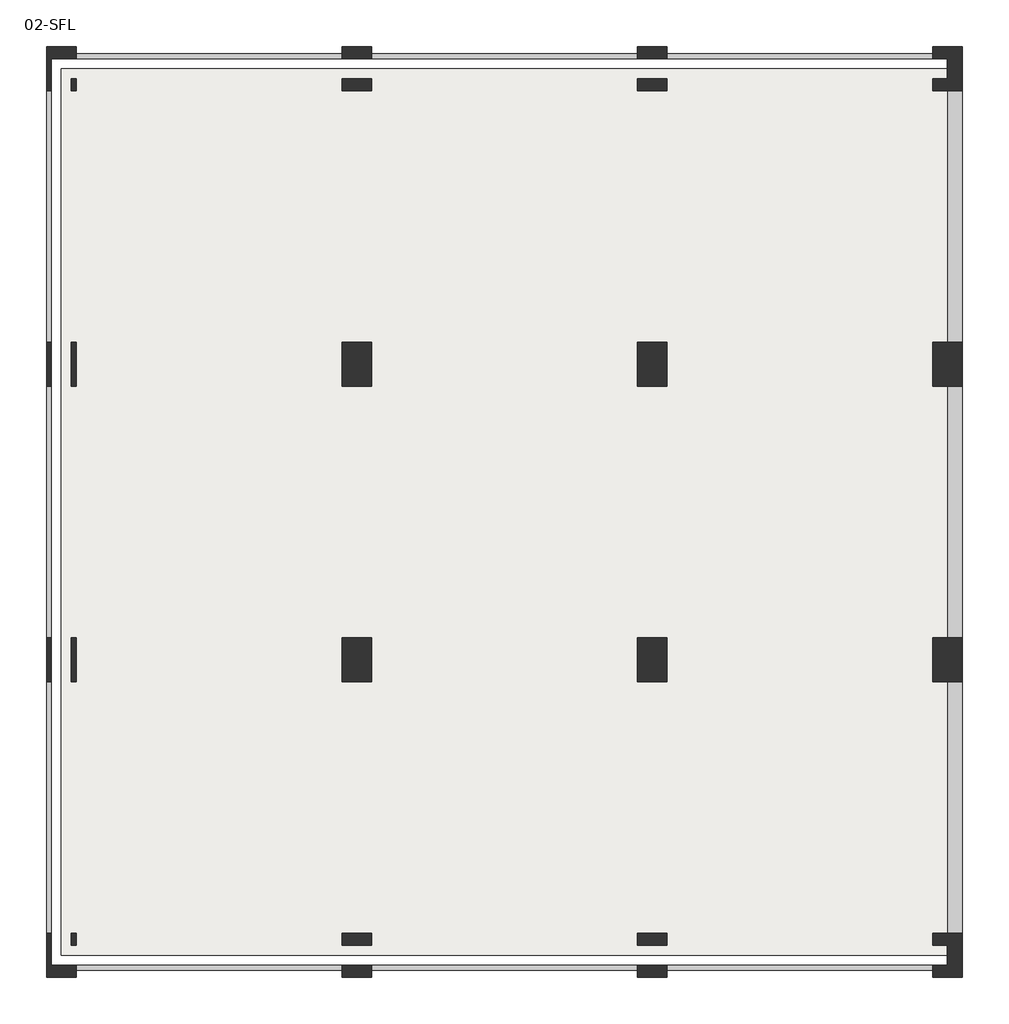
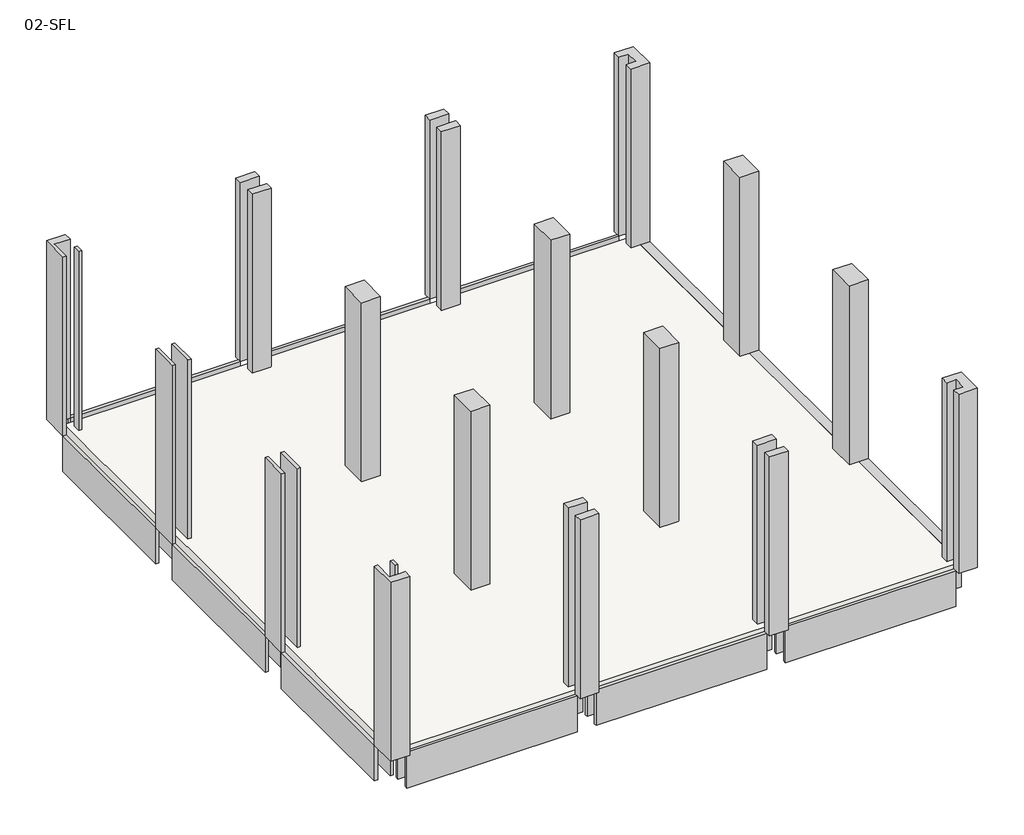
# One storey: 16 columns, 8 beams, 1 slab.
"""IFC4 building model written with IfcOpenShell, lengths in millimetres."""

from ifc_helpers import new_model, si_unit, frame, origin, place, context, project, spatial, polyline, outline, extrude, faceted_brep, element, save

model = new_model("IFC4")

# Units and contexts
model_context = context("Model", 3, world=origin())
ifc_project = project(units=[si_unit("LENGTHUNIT", "METRE", prefix="MILLI")], contexts=[model_context])

# Site, building, storey
site = spatial("IfcSite", under=ifc_project)
building = spatial("IfcBuilding", under=site)
storey = spatial("IfcBuildingStorey", under=building, Name="02-SFL", Elevation=6096.0)

# Beams
placement = place(None, origin())
element("IfcBeam", 1, ObjectType="Concrete-Rectangular Beam : 12 x 24", at=placement, inside=storey, context=model_context, shape_type="SweptSolid", body=[
    extrude(outline(polyline([(-15593.7609662, 12775.9972109), (-12850.5609662, 12775.9972109), (-12850.5609662, 12725.1972109), (-15593.7609662, 12725.1972109), (-15593.7609662, 12775.9972109)])), frame((0.0, 0.0, 5486.4), z_axis=(0.0, 0.0, 1.0), x_axis=(1.0, 0.0, 0.0)), (0.0, 0.0, 1.0), 609.6),
    extrude(outline(polyline([(-12850.5609662, 12471.1972109), (-15593.7609662, 12471.1972109), (-15593.7609662, 12521.9972109), (-12850.5609662, 12521.9972109), (-12850.5609662, 12471.1972109)])), frame((0.0, 0.0, 5486.4), z_axis=(0.0, 0.0, 1.0), x_axis=(1.0, 0.0, 0.0)), (0.0, 0.0, 1.0), 457.2),
    extrude(outline(polyline([(-18946.5609662, 12471.1972109), (-21689.7609662, 12471.1972109), (-21689.7609662, 12521.9972109), (-18946.5609662, 12521.9972109), (-18946.5609662, 12471.1972109)])), frame((0.0, 0.0, 5486.4), z_axis=(0.0, 0.0, 1.0), x_axis=(1.0, 0.0, 0.0)), (0.0, 0.0, 1.0), 457.2),
    extrude(outline(polyline([(-15898.5609662, 12471.1972109), (-18641.7609662, 12471.1972109), (-18641.7609662, 12521.9972109), (-15898.5609662, 12521.9972109), (-15898.5609662, 12471.1972109)])), frame((0.0, 0.0, 5486.4), z_axis=(0.0, 0.0, 1.0), x_axis=(1.0, 0.0, 0.0)), (0.0, 0.0, 1.0), 457.2),
    extrude(outline(polyline([(-21689.7609662, 12775.9972109), (-18946.5609662, 12775.9972109), (-18946.5609662, 12725.1972109), (-21689.7609662, 12725.1972109), (-21689.7609662, 12775.9972109)])), frame((0.0, 0.0, 5486.4), z_axis=(0.0, 0.0, 1.0), x_axis=(1.0, 0.0, 0.0)), (0.0, 0.0, 1.0), 609.6),
    extrude(outline(polyline([(-18641.7609662, 12775.9972109), (-15898.5609662, 12775.9972109), (-15898.5609662, 12725.1972109), (-18641.7609662, 12725.1972109), (-18641.7609662, 12775.9972109)])), frame((0.0, 0.0, 5486.4), z_axis=(0.0, 0.0, 1.0), x_axis=(1.0, 0.0, 0.0)), (0.0, 0.0, 1.0), 609.6),
])
element("IfcBeam", 2, ObjectType="Concrete-Rectangular Beam : 12 x 24", at=placement, inside=storey, context=model_context, shape_type="SweptSolid", body=[
    extrude(outline(polyline([(5486.4, -12850.5609662), (5486.4, -12545.7609662), (6096.0, -12545.7609662), (6096.0, -12698.1609662), (5943.6, -12698.1609662), (5943.6, -12850.5609662), (5486.4, -12850.5609662)])), frame((0.0, 3708.1972109, 0.0), z_axis=(0.0, 1.0, 0.0), x_axis=(0.0, 0.0, 1.0)), (0.0, 0.0, 1.0), 2590.8),
    extrude(outline(polyline([(5486.4, -12850.5609662), (5486.4, -12545.7609662), (6096.0, -12545.7609662), (6096.0, -12698.1609662), (5943.6, -12698.1609662), (5943.6, -12850.5609662), (5486.4, -12850.5609662)])), frame((0.0, 9804.1972109, 0.0), z_axis=(0.0, 1.0, 0.0), x_axis=(0.0, 0.0, 1.0)), (0.0, 0.0, 1.0), 2590.8),
    extrude(outline(polyline([(5486.4, -12850.5609662), (5486.4, -12545.7609662), (6096.0, -12545.7609662), (6096.0, -12698.1609662), (5943.6, -12698.1609662), (5943.6, -12850.5609662), (5486.4, -12850.5609662)])), frame((0.0, 6756.1972109, 0.0), z_axis=(0.0, 1.0, 0.0), x_axis=(0.0, 0.0, 1.0)), (0.0, 0.0, 1.0), 2590.8),
])
element("IfcBeam", 3, ObjectType="Concrete-Rectangular Beam : 12 x 24", at=placement, inside=storey, context=model_context, shape_type="SweptSolid", body=[
    extrude(outline(polyline([(-18946.5609662, 3327.1972109), (-21689.7609662, 3327.1972109), (-21689.7609662, 3377.9972109), (-18946.5609662, 3377.9972109), (-18946.5609662, 3327.1972109)])), frame((0.0, 0.0, 5486.4), z_axis=(0.0, 0.0, 1.0), x_axis=(1.0, 0.0, 0.0)), (0.0, 0.0, 1.0), 609.6),
    extrude(outline(polyline([(-21689.7609662, 3631.9972109), (-18946.5609662, 3631.9972109), (-18946.5609662, 3581.1972109), (-21689.7609662, 3581.1972109), (-21689.7609662, 3631.9972109)])), frame((0.0, 0.0, 5486.4), z_axis=(0.0, 0.0, 1.0), x_axis=(1.0, 0.0, 0.0)), (0.0, 0.0, 1.0), 457.2),
    extrude(outline(polyline([(-12850.5609662, 3327.1972109), (-15593.7609662, 3327.1972109), (-15593.7609662, 3377.9972109), (-12850.5609662, 3377.9972109), (-12850.5609662, 3327.1972109)])), frame((0.0, 0.0, 5486.4), z_axis=(0.0, 0.0, 1.0), x_axis=(1.0, 0.0, 0.0)), (0.0, 0.0, 1.0), 609.6),
    extrude(outline(polyline([(-18641.7609662, 3631.9972109), (-15898.5609662, 3631.9972109), (-15898.5609662, 3581.1972109), (-18641.7609662, 3581.1972109), (-18641.7609662, 3631.9972109)])), frame((0.0, 0.0, 5486.4), z_axis=(0.0, 0.0, 1.0), x_axis=(1.0, 0.0, 0.0)), (0.0, 0.0, 1.0), 457.2),
    extrude(outline(polyline([(-15898.5609662, 3327.1972109), (-18641.7609662, 3327.1972109), (-18641.7609662, 3377.9972109), (-15898.5609662, 3377.9972109), (-15898.5609662, 3327.1972109)])), frame((0.0, 0.0, 5486.4), z_axis=(0.0, 0.0, 1.0), x_axis=(1.0, 0.0, 0.0)), (0.0, 0.0, 1.0), 609.6),
    extrude(outline(polyline([(-15593.7609662, 3631.9972109), (-12850.5609662, 3631.9972109), (-12850.5609662, 3581.1972109), (-15593.7609662, 3581.1972109), (-15593.7609662, 3631.9972109)])), frame((0.0, 0.0, 5486.4), z_axis=(0.0, 0.0, 1.0), x_axis=(1.0, 0.0, 0.0)), (0.0, 0.0, 1.0), 457.2),
])
element("IfcBeam", 4, ObjectType="Concrete-Rectangular Beam : 12 x 24", at=placement, inside=storey, context=model_context, shape_type="SweptSolid", body=[
    extrude(outline(polyline([(-21994.5609662, 9804.1972109), (-21994.5609662, 12394.9972109), (-21943.7609662, 12394.9972109), (-21943.7609662, 9804.1972109), (-21994.5609662, 9804.1972109)])), frame((0.0, 0.0, 5486.4), z_axis=(0.0, 0.0, 1.0), x_axis=(1.0, 0.0, 0.0)), (0.0, 0.0, 1.0), 609.6),
    extrude(outline(polyline([(-21689.7609662, 12394.9972109), (-21689.7609662, 9804.1972109), (-21740.5609662, 9804.1972109), (-21740.5609662, 12394.9972109), (-21689.7609662, 12394.9972109)])), frame((0.0, 0.0, 5486.4), z_axis=(0.0, 0.0, 1.0), x_axis=(1.0, 0.0, 0.0)), (0.0, 0.0, 1.0), 457.2),
    extrude(outline(polyline([(-21689.7609662, 6298.9972109), (-21689.7609662, 3708.1972109), (-21740.5609662, 3708.1972109), (-21740.5609662, 6298.9972109), (-21689.7609662, 6298.9972109)])), frame((0.0, 0.0, 5486.4), z_axis=(0.0, 0.0, 1.0), x_axis=(1.0, 0.0, 0.0)), (0.0, 0.0, 1.0), 457.2),
    extrude(outline(polyline([(-21689.7609662, 9346.9972109), (-21689.7609662, 6756.1972109), (-21740.5609662, 6756.1972109), (-21740.5609662, 9346.9972109), (-21689.7609662, 9346.9972109)])), frame((0.0, 0.0, 5486.4), z_axis=(0.0, 0.0, 1.0), x_axis=(1.0, 0.0, 0.0)), (0.0, 0.0, 1.0), 457.2),
    extrude(outline(polyline([(-21994.5609662, 6756.1972109), (-21994.5609662, 9346.9972109), (-21943.7609662, 9346.9972109), (-21943.7609662, 6756.1972109), (-21994.5609662, 6756.1972109)])), frame((0.0, 0.0, 5486.4), z_axis=(0.0, 0.0, 1.0), x_axis=(1.0, 0.0, 0.0)), (0.0, 0.0, 1.0), 609.6),
    extrude(outline(polyline([(-21994.5609662, 3708.1972109), (-21994.5609662, 6298.9972109), (-21943.7609662, 6298.9972109), (-21943.7609662, 3708.1972109), (-21994.5609662, 3708.1972109)])), frame((0.0, 0.0, 5486.4), z_axis=(0.0, 0.0, 1.0), x_axis=(1.0, 0.0, 0.0)), (0.0, 0.0, 1.0), 609.6),
])
element("IfcBeam", 5, ObjectType="Concrete-Rectangular Beam : 12 x 24", at=placement, inside=storey, context=model_context, shape_type="SweptSolid", body=[
    extrude(outline(polyline([(-12850.5609662, 9727.9972109), (-12850.5609662, 9423.1972109), (-15593.7609662, 9423.1972109), (-15593.7609662, 9727.9972109), (-12850.5609662, 9727.9972109)])), frame((0.0, 0.0, 5486.4), z_axis=(0.0, 0.0, 1.0), x_axis=(1.0, 0.0, 0.0)), (0.0, 0.0, 1.0), 457.2),
    extrude(outline(polyline([(-21689.7609662, 9423.1972109), (-21689.7609662, 9727.9972109), (-18946.5609662, 9727.9972109), (-18946.5609662, 9423.1972109), (-21689.7609662, 9423.1972109)])), frame((0.0, 0.0, 5486.4), z_axis=(0.0, 0.0, 1.0), x_axis=(1.0, 0.0, 0.0)), (0.0, 0.0, 1.0), 457.2),
    extrude(outline(polyline([(-18641.7609662, 9423.1972109), (-18641.7609662, 9727.9972109), (-15898.5609662, 9727.9972109), (-15898.5609662, 9423.1972109), (-18641.7609662, 9423.1972109)])), frame((0.0, 0.0, 5486.4), z_axis=(0.0, 0.0, 1.0), x_axis=(1.0, 0.0, 0.0)), (0.0, 0.0, 1.0), 457.2),
])
element("IfcBeam", 6, ObjectType="Concrete-Rectangular Beam : 12 x 24", at=placement, inside=storey, context=model_context, shape_type="SweptSolid", body=[
    extrude(outline(polyline([(-12850.5609662, 6679.9972109), (-12850.5609662, 6375.1972109), (-15593.7609662, 6375.1972109), (-15593.7609662, 6679.9972109), (-12850.5609662, 6679.9972109)])), frame((0.0, 0.0, 5486.4), z_axis=(0.0, 0.0, 1.0), x_axis=(1.0, 0.0, 0.0)), (0.0, 0.0, 1.0), 457.2),
    extrude(outline(polyline([(-21689.7609662, 6375.1972109), (-21689.7609662, 6679.9972109), (-18946.5609662, 6679.9972109), (-18946.5609662, 6375.1972109), (-21689.7609662, 6375.1972109)])), frame((0.0, 0.0, 5486.4), z_axis=(0.0, 0.0, 1.0), x_axis=(1.0, 0.0, 0.0)), (0.0, 0.0, 1.0), 457.2),
    extrude(outline(polyline([(-18641.7609662, 6375.1972109), (-18641.7609662, 6679.9972109), (-15898.5609662, 6679.9972109), (-15898.5609662, 6375.1972109), (-18641.7609662, 6375.1972109)])), frame((0.0, 0.0, 5486.4), z_axis=(0.0, 0.0, 1.0), x_axis=(1.0, 0.0, 0.0)), (0.0, 0.0, 1.0), 457.2),
])
element("IfcBeam", 7, ObjectType="Concrete-Rectangular Beam : 12 x 24", at=placement, inside=storey, context=model_context, shape_type="SweptSolid", body=[
    extrude(outline(polyline([(-18641.7609662, 3708.1972109), (-18946.5609662, 3708.1972109), (-18946.5609662, 6298.9972109), (-18641.7609662, 6298.9972109), (-18641.7609662, 3708.1972109)])), frame((0.0, 0.0, 5486.4), z_axis=(0.0, 0.0, 1.0), x_axis=(1.0, 0.0, 0.0)), (0.0, 0.0, 1.0), 457.2),
    extrude(outline(polyline([(-18946.5609662, 12394.9972109), (-18641.7609662, 12394.9972109), (-18641.7609662, 9804.1972109), (-18946.5609662, 9804.1972109), (-18946.5609662, 12394.9972109)])), frame((0.0, 0.0, 5486.4), z_axis=(0.0, 0.0, 1.0), x_axis=(1.0, 0.0, 0.0)), (0.0, 0.0, 1.0), 457.2),
    extrude(outline(polyline([(-18946.5609662, 9346.9972109), (-18641.7609662, 9346.9972109), (-18641.7609662, 6756.1972109), (-18946.5609662, 6756.1972109), (-18946.5609662, 9346.9972109)])), frame((0.0, 0.0, 5486.4), z_axis=(0.0, 0.0, 1.0), x_axis=(1.0, 0.0, 0.0)), (0.0, 0.0, 1.0), 457.2),
])
element("IfcBeam", 8, ObjectType="Concrete-Rectangular Beam : 12 x 24", at=placement, inside=storey, context=model_context, shape_type="SweptSolid", body=[
    extrude(outline(polyline([(-15593.7609662, 3708.1972109), (-15898.5609662, 3708.1972109), (-15898.5609662, 6298.9972109), (-15593.7609662, 6298.9972109), (-15593.7609662, 3708.1972109)])), frame((0.0, 0.0, 5486.4), z_axis=(0.0, 0.0, 1.0), x_axis=(1.0, 0.0, 0.0)), (0.0, 0.0, 1.0), 457.2),
    extrude(outline(polyline([(-15898.5609662, 12394.9972109), (-15593.7609662, 12394.9972109), (-15593.7609662, 9804.1972109), (-15898.5609662, 9804.1972109), (-15898.5609662, 12394.9972109)])), frame((0.0, 0.0, 5486.4), z_axis=(0.0, 0.0, 1.0), x_axis=(1.0, 0.0, 0.0)), (0.0, 0.0, 1.0), 457.2),
    extrude(outline(polyline([(-15898.5609662, 9346.9972109), (-15593.7609662, 9346.9972109), (-15593.7609662, 6756.1972109), (-15898.5609662, 6756.1972109), (-15898.5609662, 9346.9972109)])), frame((0.0, 0.0, 5486.4), z_axis=(0.0, 0.0, 1.0), x_axis=(1.0, 0.0, 0.0)), (0.0, 0.0, 1.0), 457.2),
])

# Columns
element("IfcColumn", 9, ObjectType="Concrete-Rectangular-Column : 12 x 18", at=placement, inside=storey, context=model_context, shape_type="Brep", body=[
    faceted_brep([(-21689.7609662, 12521.9972109, 6096.0), (-21689.7609662, 12394.9972109, 6096.0), (-21740.5609662, 12394.9972109, 6096.0), (-21740.5609662, 12521.9972109, 6096.0), (-21689.7609662, 12394.9972109, 9144.0), (-21689.7609662, 12521.9972109, 9144.0), (-21740.5609662, 12394.9972109, 9144.0), (-21740.5609662, 12521.9972109, 9144.0)], [[[0, 1, 2, 3]], [[4, 1, 0, 5]], [[1, 4, 6, 2]], [[5, 0, 3, 7]], [[3, 2, 6, 7]], [[4, 5, 7, 6]]]),
    faceted_brep([(-21994.5609662, 12852.1972109, 6096.0), (-21994.5609662, 12394.9972109, 6096.0), (-21994.5609662, 12394.9972109, 9144.0), (-21994.5609662, 12852.1972109, 9144.0), (-21689.7609662, 12852.1972109, 6096.0), (-21689.7609662, 12852.1972109, 9144.0), (-21943.7609662, 12394.9972109, 9144.0), (-21943.7609662, 12521.9972109, 9144.0), (-21943.7609662, 12725.1972109, 9144.0), (-21689.7609662, 12725.1972109, 9144.0), (-21943.7609662, 12725.1972109, 6096.0), (-21689.7609662, 12725.1972109, 6096.0), (-21943.7609662, 12394.9972109, 6096.0)], [[[0, 1, 2, 3]], [[4, 0, 3, 5]], [[3, 2, 6, 7, 8, 9, 5]], [[10, 11, 9, 8]], [[4, 5, 9, 11]], [[10, 8, 7, 6, 12]], [[1, 0, 4, 11, 10, 12]], [[2, 1, 12, 6]]]),
])
element("IfcColumn", 10, ObjectType="Concrete-Rectangular-Column : 12 x 18", at=placement, inside=storey, context=model_context, shape_type="SweptSolid", body=[
    extrude(outline(polyline([(-21689.7609662, 9804.1972109), (-21689.7609662, 9346.9972109), (-21740.5609662, 9346.9972109), (-21740.5609662, 9804.1972109), (-21689.7609662, 9804.1972109)])), frame((0.0, 0.0, 6096.0), z_axis=(0.0, 0.0, 1.0), x_axis=(1.0, 0.0, 0.0)), (0.0, 0.0, 1.0), 3048.0),
    extrude(outline(polyline([(-21994.5609662, 9346.9972109), (-21994.5609662, 9804.1972109), (-21943.7609662, 9804.1972109), (-21943.7609662, 9346.9972109), (-21994.5609662, 9346.9972109)])), frame((0.0, 0.0, 6096.0), z_axis=(0.0, 0.0, 1.0), x_axis=(1.0, 0.0, 0.0)), (0.0, 0.0, 1.0), 3048.0),
])
element("IfcColumn", 11, ObjectType="Concrete-Rectangular-Column : 12 x 18", at=placement, inside=storey, context=model_context, shape_type="SweptSolid", body=[
    extrude(outline(polyline([(-21689.7609662, 6756.1972109), (-21689.7609662, 6298.9972109), (-21740.5609662, 6298.9972109), (-21740.5609662, 6756.1972109), (-21689.7609662, 6756.1972109)])), frame((0.0, 0.0, 6096.0), z_axis=(0.0, 0.0, 1.0), x_axis=(1.0, 0.0, 0.0)), (0.0, 0.0, 1.0), 3048.0),
    extrude(outline(polyline([(-21994.5609662, 6298.9972109), (-21994.5609662, 6756.1972109), (-21943.7609662, 6756.1972109), (-21943.7609662, 6298.9972109), (-21994.5609662, 6298.9972109)])), frame((0.0, 0.0, 6096.0), z_axis=(0.0, 0.0, 1.0), x_axis=(1.0, 0.0, 0.0)), (0.0, 0.0, 1.0), 3048.0),
])
element("IfcColumn", 12, ObjectType="Concrete-Rectangular-Column : 12 x 18", at=placement, inside=storey, context=model_context, shape_type="Brep", body=[
    faceted_brep([(-21740.5609662, 3708.1972109, 6096.0), (-21689.7609662, 3708.1972109, 6096.0), (-21689.7609662, 3581.1972109, 6096.0), (-21740.5609662, 3581.1972109, 6096.0), (-21689.7609662, 3708.1972109, 9144.0), (-21740.5609662, 3708.1972109, 9144.0), (-21740.5609662, 3581.1972109, 9144.0), (-21689.7609662, 3581.1972109, 9144.0)], [[[0, 1, 2, 3]], [[4, 1, 0, 5]], [[5, 0, 3, 6]], [[3, 2, 7, 6]], [[1, 4, 7, 2]], [[4, 5, 6, 7]]]),
    faceted_brep([(-21994.5609662, 3708.1972109, 6096.0), (-21994.5609662, 3250.9972109, 6096.0), (-21994.5609662, 3250.9972109, 9144.0), (-21994.5609662, 3708.1972109, 9144.0), (-21689.7609662, 3250.9972109, 9144.0), (-21689.7609662, 3250.9972109, 6096.0), (-21689.7609662, 3377.9972109, 6096.0), (-21689.7609662, 3377.9972109, 9144.0), (-21740.5609662, 3377.9972109, 9144.0), (-21943.7609662, 3377.9972109, 9144.0), (-21943.7609662, 3708.1972109, 9144.0), (-21943.7609662, 3377.9972109, 6096.0), (-21943.7609662, 3708.1972109, 6096.0)], [[[0, 1, 2, 3]], [[4, 5, 6, 7]], [[1, 5, 4, 2]], [[3, 2, 4, 7, 8, 9, 10]], [[11, 12, 10, 9]], [[0, 3, 10, 12]], [[11, 9, 8, 7, 6]], [[1, 0, 12, 11, 6, 5]]]),
])
element("IfcColumn", 13, ObjectType="Concrete-Rectangular-Column : 12 x 18", at=placement, inside=storey, context=model_context, shape_type="SweptSolid", body=[
    extrude(outline(polyline([(-18641.7609662, 12394.9972109), (-18946.5609662, 12394.9972109), (-18946.5609662, 12521.9972109), (-18641.7609662, 12521.9972109), (-18641.7609662, 12394.9972109)])), frame((0.0, 0.0, 6096.0), z_axis=(0.0, 0.0, 1.0), x_axis=(1.0, 0.0, 0.0)), (0.0, 0.0, 1.0), 3048.0),
    extrude(outline(polyline([(-18946.5609662, 12852.1972109), (-18641.7609662, 12852.1972109), (-18641.7609662, 12725.1972109), (-18946.5609662, 12725.1972109), (-18946.5609662, 12852.1972109)])), frame((0.0, 0.0, 6096.0), z_axis=(0.0, 0.0, 1.0), x_axis=(1.0, 0.0, 0.0)), (0.0, 0.0, 1.0), 3048.0),
])
element("IfcColumn", 14, ObjectType="Concrete-Rectangular-Column : 12 x 18", at=placement, inside=storey, context=model_context, shape_type="SweptSolid", body=[
    extrude(outline(polyline([(-18946.5609662, 9346.9972109), (-18946.5609662, 9804.1972109), (-18641.7609662, 9804.1972109), (-18641.7609662, 9346.9972109), (-18946.5609662, 9346.9972109)])), frame((0.0, 0.0, 6096.0), z_axis=(0.0, 0.0, 1.0), x_axis=(1.0, 0.0, 0.0)), (0.0, 0.0, 1.0), 3048.0),
])
element("IfcColumn", 15, ObjectType="Concrete-Rectangular-Column : 12 x 18", at=placement, inside=storey, context=model_context, shape_type="SweptSolid", body=[
    extrude(outline(polyline([(-18946.5609662, 6298.9972109), (-18946.5609662, 6756.1972109), (-18641.7609662, 6756.1972109), (-18641.7609662, 6298.9972109), (-18946.5609662, 6298.9972109)])), frame((0.0, 0.0, 6096.0), z_axis=(0.0, 0.0, 1.0), x_axis=(1.0, 0.0, 0.0)), (0.0, 0.0, 1.0), 3048.0),
])
element("IfcColumn", 16, ObjectType="Concrete-Rectangular-Column : 12 x 18", at=placement, inside=storey, context=model_context, shape_type="SweptSolid", body=[
    extrude(outline(polyline([(-18641.7609662, 3250.9972109), (-18946.5609662, 3250.9972109), (-18946.5609662, 3377.9972109), (-18641.7609662, 3377.9972109), (-18641.7609662, 3250.9972109)])), frame((0.0, 0.0, 6096.0), z_axis=(0.0, 0.0, 1.0), x_axis=(1.0, 0.0, 0.0)), (0.0, 0.0, 1.0), 3048.0),
    extrude(outline(polyline([(-18946.5609662, 3708.1972109), (-18641.7609662, 3708.1972109), (-18641.7609662, 3581.1972109), (-18946.5609662, 3581.1972109), (-18946.5609662, 3708.1972109)])), frame((0.0, 0.0, 6096.0), z_axis=(0.0, 0.0, 1.0), x_axis=(1.0, 0.0, 0.0)), (0.0, 0.0, 1.0), 3048.0),
])
element("IfcColumn", 17, ObjectType="Concrete-Rectangular-Column : 12 x 18", at=placement, inside=storey, context=model_context, shape_type="SweptSolid", body=[
    extrude(outline(polyline([(-15593.7609662, 12394.9972109), (-15898.5609662, 12394.9972109), (-15898.5609662, 12521.9972109), (-15593.7609662, 12521.9972109), (-15593.7609662, 12394.9972109)])), frame((0.0, 0.0, 6096.0), z_axis=(0.0, 0.0, 1.0), x_axis=(1.0, 0.0, 0.0)), (0.0, 0.0, 1.0), 3048.0),
    extrude(outline(polyline([(-15898.5609662, 12852.1972109), (-15593.7609662, 12852.1972109), (-15593.7609662, 12725.1972109), (-15898.5609662, 12725.1972109), (-15898.5609662, 12852.1972109)])), frame((0.0, 0.0, 6096.0), z_axis=(0.0, 0.0, 1.0), x_axis=(1.0, 0.0, 0.0)), (0.0, 0.0, 1.0), 3048.0),
])
element("IfcColumn", 18, ObjectType="Concrete-Rectangular-Column : 12 x 18", at=placement, inside=storey, context=model_context, shape_type="SweptSolid", body=[
    extrude(outline(polyline([(-15898.5609662, 9346.9972109), (-15898.5609662, 9804.1972109), (-15593.7609662, 9804.1972109), (-15593.7609662, 9346.9972109), (-15898.5609662, 9346.9972109)])), frame((0.0, 0.0, 6096.0), z_axis=(0.0, 0.0, 1.0), x_axis=(1.0, 0.0, 0.0)), (0.0, 0.0, 1.0), 3048.0),
])
element("IfcColumn", 19, ObjectType="Concrete-Rectangular-Column : 12 x 18", at=placement, inside=storey, context=model_context, shape_type="SweptSolid", body=[
    extrude(outline(polyline([(-15898.5609662, 6298.9972109), (-15898.5609662, 6756.1972109), (-15593.7609662, 6756.1972109), (-15593.7609662, 6298.9972109), (-15898.5609662, 6298.9972109)])), frame((0.0, 0.0, 6096.0), z_axis=(0.0, 0.0, 1.0), x_axis=(1.0, 0.0, 0.0)), (0.0, 0.0, 1.0), 3048.0),
])
element("IfcColumn", 20, ObjectType="Concrete-Rectangular-Column : 12 x 18", at=placement, inside=storey, context=model_context, shape_type="SweptSolid", body=[
    extrude(outline(polyline([(-15593.7609662, 3250.9972109), (-15898.5609662, 3250.9972109), (-15898.5609662, 3377.9972109), (-15593.7609662, 3377.9972109), (-15593.7609662, 3250.9972109)])), frame((0.0, 0.0, 6096.0), z_axis=(0.0, 0.0, 1.0), x_axis=(1.0, 0.0, 0.0)), (0.0, 0.0, 1.0), 3048.0),
    extrude(outline(polyline([(-15898.5609662, 3708.1972109), (-15593.7609662, 3708.1972109), (-15593.7609662, 3581.1972109), (-15898.5609662, 3581.1972109), (-15898.5609662, 3708.1972109)])), frame((0.0, 0.0, 6096.0), z_axis=(0.0, 0.0, 1.0), x_axis=(1.0, 0.0, 0.0)), (0.0, 0.0, 1.0), 3048.0),
])
element("IfcColumn", 21, ObjectType="Concrete-Rectangular-Column : 12 x 18", at=placement, inside=storey, context=model_context, shape_type="SweptSolid", body=[
    extrude(outline(polyline([(-12850.5609662, 12852.1972109), (-12545.7609662, 12852.1972109), (-12545.7609662, 12394.9972109), (-12850.5609662, 12394.9972109), (-12850.5609662, 12521.9972109), (-12698.1609662, 12521.9972109), (-12698.1609662, 12725.1972109), (-12850.5609662, 12725.1972109), (-12850.5609662, 12852.1972109)])), frame((0.0, 0.0, 6096.0), z_axis=(0.0, 0.0, 1.0), x_axis=(1.0, 0.0, 0.0)), (0.0, 0.0, 1.0), 3048.0),
])
element("IfcColumn", 22, ObjectType="Concrete-Rectangular-Column : 12 x 18", at=placement, inside=storey, context=model_context, shape_type="SweptSolid", body=[
    extrude(outline(polyline([(-12850.5609662, 9346.9972109), (-12850.5609662, 9804.1972109), (-12545.7609662, 9804.1972109), (-12545.7609662, 9346.9972109), (-12850.5609662, 9346.9972109)])), frame((0.0, 0.0, 6096.0), z_axis=(0.0, 0.0, 1.0), x_axis=(1.0, 0.0, 0.0)), (0.0, 0.0, 1.0), 3048.0),
])
element("IfcColumn", 23, ObjectType="Concrete-Rectangular-Column : 12 x 18", at=placement, inside=storey, context=model_context, shape_type="SweptSolid", body=[
    extrude(outline(polyline([(-12850.5609662, 6298.9972109), (-12850.5609662, 6756.1972109), (-12545.7609662, 6756.1972109), (-12545.7609662, 6298.9972109), (-12850.5609662, 6298.9972109)])), frame((0.0, 0.0, 6096.0), z_axis=(0.0, 0.0, 1.0), x_axis=(1.0, 0.0, 0.0)), (0.0, 0.0, 1.0), 3048.0),
])
element("IfcColumn", 24, ObjectType="Concrete-Rectangular-Column : 12 x 18", at=placement, inside=storey, context=model_context, shape_type="SweptSolid", body=[
    extrude(outline(polyline([(-12850.5609662, 3708.1972109), (-12545.7609662, 3708.1972109), (-12545.7609662, 3250.9972109), (-12850.5609662, 3250.9972109), (-12850.5609662, 3377.9972109), (-12698.1609662, 3377.9972109), (-12698.1609662, 3581.1972109), (-12850.5609662, 3581.1972109), (-12850.5609662, 3708.1972109)])), frame((0.0, 0.0, 6096.0), z_axis=(0.0, 0.0, 1.0), x_axis=(1.0, 0.0, 0.0)), (0.0, 0.0, 1.0), 3048.0),
])

# Slab
element("IfcSlab", 25, ObjectType="6\" Foundation Slab", at=placement, inside=storey, context=model_context, shape_type="Brep", body=[
    faceted_brep([(-12698.1609662, 12623.5972109, 5943.6), (-12698.1609662, 12394.9972109, 5943.6), (-12698.1609662, 9804.1972109, 5943.6), (-12698.1609662, 9346.9972109, 5943.6), (-12698.1609662, 6756.1972109, 5943.6), (-12698.1609662, 6298.9972109, 5943.6), (-12698.1609662, 3708.1972109, 5943.6), (-12698.1609662, 3479.5972109, 5943.6), (-21842.1609662, 3479.5972109, 5943.6), (-21842.1609662, 12623.5972109, 5943.6), (-12698.1609662, 12623.5972109, 6096.0), (-21842.1609662, 12623.5972109, 6096.0), (-21842.1609662, 3479.5972109, 6096.0), (-12698.1609662, 3479.5972109, 6096.0), (-12698.1609662, 3708.1972109, 6096.0), (-12698.1609662, 6298.9972109, 6096.0), (-12698.1609662, 6756.1972109, 6096.0), (-12698.1609662, 9346.9972109, 6096.0), (-12698.1609662, 9804.1972109, 6096.0), (-12698.1609662, 12394.9972109, 6096.0)], [[[0, 1, 2, 3, 4, 5, 6, 7, 8, 9]], [[10, 11, 12, 13, 14, 15, 16, 17, 18, 19]], [[7, 6, 5, 4, 3, 2, 1, 0, 10, 19, 18, 17, 16, 15, 14, 13]], [[8, 7, 13, 12]], [[9, 8, 12, 11]], [[0, 9, 11, 10]]]),
])

save(model, "model.ifc")

# Revit data of these elements
# Type "Concrete-Rectangular Beam : 12 x 24"
#   Assembly Code = "B10"
#   Length [instance default] = 5' - 0"
#   b = 1' - 0"
#   h = 2' - 0"
#   Structural Material [instance default] = Concrete, Cast-in-Place gray
# Type "Concrete-Rectangular-Column : 12 x 18"
#   Assembly Code = "B10"
#   b = 1' - 0"
#   h = 1' - 6"
#   Structural Material [instance default] = Concrete, Cast-in-Place gray
# Type "6\" Foundation Slab"
#   Layers, outside or top first: 0' - 6" "Concrete, Cast-in-Place gray" (function 1)
# Elements 1, 2, 3, 4, 5, 6, 7, 8 (IfcBeam, "Concrete-Rectangular Beam : 12 x 24")
#   Structural Material = Concrete, Cast-in-Place gray
#   Phase Created = New Construction
#   Materials on its faces: "Concrete, Cast-in-Place gray"
# Elements 9, 10, 11, 12, 13, 14, 15, 16, 17, 18, 19, 20, 21, 22, 23, 24 (IfcColumn, "Concrete-Rectangular-Column : 12 x 18")
#   Comments = ""
#   Structural Material = Concrete, Cast-in-Place gray
#   Phase Created = New Construction
#   Materials on its faces: "Concrete, Cast-in-Place gray"
# Element 25 (IfcSlab, "6\" Foundation Slab")
#   Height Offset From Level = 0' - 0"
#   built-in parameter 1001954 = 1
#   Phase Created = New Construction
#   Materials on its faces: "Concrete, Cast-in-Place gray"
# Materials
#   "Concrete, Cast-in-Place gray": class "Concrete", colour RGB 192 192 192, transparency 0, Description = "Cast-in-place concrete", Cost = 0
